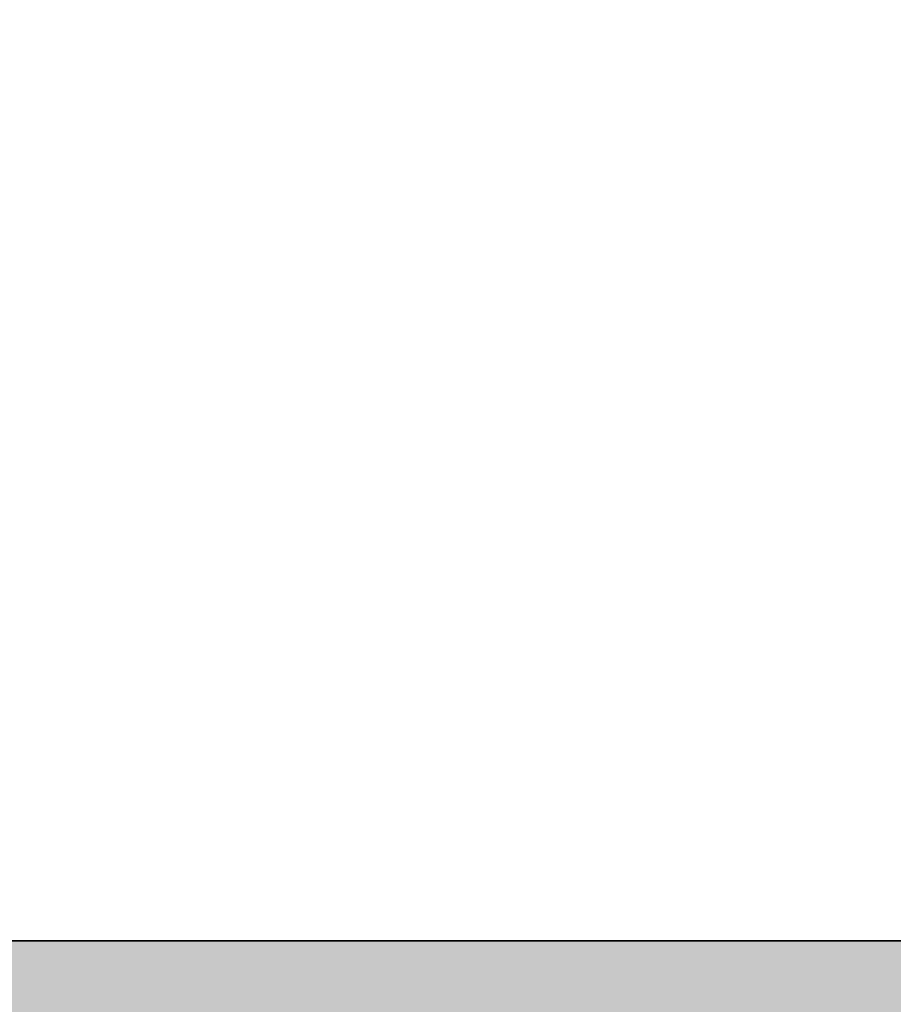
# Model space of a CAD drawing. Units: inches. Extents: x 2083 to 3317, y 1141 to 2115.
# Tile 27 of 256: x 2235.9182 to 2235.95532, y 1477.75866 to 1477.8005. Entities that reach past the tile are written whole.
import ezdxf

# ---------------------------------------------------------------- set-up
doc = ezdxf.new("R2010")
doc.units = ezdxf.units.IN
doc.layers.add('A-ANNO-DIMS', color=2, linetype='Continuous', lineweight=18)
doc.layers.add('A-WALL', color=7, linetype='Continuous', lineweight=35)
doc.layers.add('A-WALL-PATT', color=251, linetype='Continuous', lineweight=13, true_color=0x636466)
doc.styles.get("Standard").update_dxf_attribs({"font": 'arial.ttf'})
doc.dimstyles.new('ISO-25', dxfattribs={"dimtxt": 12, "dimasz": 12, "dimexe": 1.25, "dimexo": 0.625, "dimtad": 1, "dimlunit": 3, "dimtxsty": 'Standard', "dimcen": 2.5, "dimadec": 0, "dimazin": 0, "dimtfac": 1, "dimtmove": 0, "dimatfit": 3, "dimfxl": 1, "dimarcsym": 0})

# ---------------------------------------------------------------- blocks, each defined once
blk = doc.blocks.new('*D30')
at = {"layer": 'A-ANNO-DIMS', "color": 0, "lineweight": -2, "transparency": 16777216}
for p, q in [((2240.017856, 1445.273807), (2240.017856, 1448.045528)), ((2254.329327, 1445.273807), (2254.329327, 1448.045528)), ((2228.017856, 1446.795528), (2216.017856, 1446.795528)), ((2240.017856, 1446.795528), (2254.329327, 1446.795528)), ((2266.329327, 1446.795528), (2413.764866, 1446.795528))]:
    blk.add_line(p, q, dxfattribs=at)
at = {"layer": 'A-ANNO-DIMS', "color": 0, "transparency": 16777216}
for points in [[(2228.017856, 1448.795528), (2228.017856, 1444.795528), (2240.017856, 1446.795528)], [(2266.329327, 1448.795528), (2266.329327, 1444.795528), (2254.329327, 1446.795528)]]:
    blk.add_solid(points, dxfattribs=at)
at = {"layer": 'Defpoints', "color": 0, "transparency": 16777216}
for p in [(2254.329327, 1446.795528), (2240.017856, 1444.648807), (2254.329327, 1444.648807)]:
    blk.add_point(p, dxfattribs=at)
at = {"layer": 'A-ANNO-DIMS', "color": 0, "transparency": 16777216, "insert": (2346.047096, 1453.625167), "char_height": 12, "attachment_point": 5}
blk.add_mtext('WC 1\'-2 1/2" TYP.', dxfattribs=at)
blk = doc.blocks.new('*D31')
at = {"layer": 'A-ANNO-DIMS', "color": 0, "lineweight": -2, "transparency": 16777216}
for p, q in [((2237.871136, 1456.648807), (2237.871136, 1541.915179)), ((2239.392856, 1444.648807), (2236.621136, 1444.648807)), ((2237.871136, 1431.547542), (2237.871136, 1444.648807)), ((2239.392856, 1431.547542), (2236.621136, 1431.547542)), ((2237.871136, 1419.547542), (2237.871136, 1407.547542))]:
    blk.add_line(p, q, dxfattribs=at)
at = {"layer": 'A-ANNO-DIMS', "color": 0, "transparency": 16777216}
for points in [[(2235.871136, 1456.648807), (2239.871136, 1456.648807), (2237.871136, 1444.648807)], [(2235.871136, 1419.547542), (2239.871136, 1419.547542), (2237.871136, 1431.547542)]]:
    blk.add_solid(points, dxfattribs=at)
at = {"layer": 'Defpoints', "color": 0, "transparency": 16777216}
for p in [(2237.871136, 1444.648807), (2240.017856, 1444.648807), (2240.017856, 1431.547542)]:
    blk.add_point(p, dxfattribs=at)
at = {"layer": 'A-ANNO-DIMS', "color": 0, "transparency": 16777216, "insert": (2231.217486, 1505.281993), "char_height": 12, "attachment_point": 5, "rotation": 90}
blk.add_mtext('1\'-1" TYP.', dxfattribs=at)

msp = doc.modelspace()

# ---------------------------------------------------------------- hatches: boundary and pattern name
at = {"layer": 'A-WALL-PATT'}
h = msp.add_hatch(color=256, dxfattribs=at)
h.dxf.hatch_style = 1
h.paths.add_polyline_path([(3126.959783, 2020.76136), (2748.959783, 2020.76136), (2604.959783, 2020.76136), (2226.959783, 2020.76136), (2226.959783, 1702.76136), (2466.959783, 1702.76136), (2466.959783, 1582.76136), (2418.959783, 1582.76136), (2418.959783, 1477.76136), (2226.959783, 1477.76136), (2226.959783, 1263.26136), (2544.959783, 1263.26136), (2544.959783, 1411.76136), (2604.959783, 1411.76136), (2685.959783, 1411.76136), (2685.959783, 1420.76136), (2604.959783, 1420.76136), (2604.959783, 1573.76136), (2604.959783, 1702.76136), (2604.959783, 2011.76136), (2748.959783, 2011.76136), (2748.959783, 1702.76136), (2862.959783, 1702.76136), (2862.959783, 1621.76136), (2871.959783, 1621.76136), (2871.959783, 1702.76136), (2883.959783, 1702.76136), (2883.959783, 1706.939459, -0.026459), (2883.959783, 1711.76136), (2757.959783, 1711.76136), (2757.959783, 1807.76136), (2787.959783, 1807.76136), (2787.959783, 1812.26136), (2757.959783, 1812.26136), (2757.959783, 2011.76136), (2877.959783, 2011.76136), (2877.959783, 1812.26136), (2847.959783, 1812.26136), (2847.959783, 1807.76136), (2889.835742, 1807.76136), (2889.835742, 1812.26136), (2882.459783, 1812.26136), (2882.459783, 2011.76136), (3117.959783, 2011.76136), (3117.959783, 1812.26136), (2937.835742, 1812.26136), (2937.835742, 1807.76136), (2995.709783, 1807.76136), (2995.709783, 1796.117666), (3000.209783, 1796.117666), (3000.209783, 1807.76136), (3117.959783, 1807.76136), (3117.959783, 1711.76136), (3000.209783, 1711.76136), (3000.209783, 1760.117666), (2998.572705, 1760.117666, -0.020711), (2995.709783, 1760.117666), (2995.709783, 1711.76136), (2931.959783, 1711.76136), (2931.959783, 1702.76136), (3126.959783, 1702.76136)])
h.paths.add_polyline_path([(2471.459783, 2011.76136), (2471.459783, 1810.01136), (2462.716936, 1810.01136), (2462.716936, 1805.51136), (2505.959783, 1805.51136), (2505.959783, 1810.01136), (2475.959783, 1810.01136), (2475.959783, 2011.76136), (2595.959783, 2011.76136), (2595.959783, 1810.01136), (2565.959783, 1810.01136), (2565.959783, 1805.51136), (2595.959783, 1805.51136), (2595.959783, 1711.76136), (2235.959783, 1711.76136), (2235.959783, 1805.51136), (2353.709783, 1805.51136), (2353.709783, 1796.054162), (2358.209783, 1796.054162), (2358.209783, 1805.51136), (2414.716936, 1805.51136), (2414.716936, 1810.01136), (2235.959783, 1810.01136), (2235.959783, 2011.76136)], flags=16)
h.paths.add_polyline_path([(2270.204734, 1994.610008), (2270.204734, 1970.610008), (2246.204734, 1970.610008), (2246.204734, 1994.610008)], flags=0)
edge = h.paths.add_edge_path(flags=0)
edge.add_ellipse((2332.027391, 1899.798176), major_axis=(-3.042994, 3.042994), ratio=0.16825245, start_angle=-161.332166, end_angle=-156.307114, ccw=False)
edge.add_ellipse((2333.082037, 1898.74353), major_axis=(-1.054646, 1.054646), ratio=0.4535321, start_angle=-123.371019, end_angle=-94.159107)
edge = h.paths.add_edge_path(flags=0)
edge.add_ellipse((2332.027391, 1968.87629), major_axis=(3.042994, 3.042994), ratio=0.16825245, start_angle=18.667834, end_angle=23.692886)
edge.add_spline(control_points=[(2332.925596, 1970.691105), (2332.226768, 1970.3361), (2330.893709, 1969.658905), (2328.41308, 1970.932138), (2327.203934, 1967.748712), (2324.709596, 1969.955589), (2322.532822, 1967.012354), (2320.012846, 1971.295812), (2317.680308, 1968.157845), (2316.040526, 1967.102047), (2315.426904, 1966.809602)], knot_values=[0, 0, 0, 0, 2.267059, 4.324559, 6.685584, 8.878641, 11.121502, 14.300359, 17.755284, 19.732645, 19.732645, 19.732645, 19.732645], degree=3, periodic=0)
edge.add_ellipse((2332.027391, 1968.87629), major_axis=(3.042994, 3.042994), ratio=0.16825245, start_angle=18.667834, end_angle=23.692886, ccw=False)
edge.add_ellipse((2333.082037, 1969.930936), major_axis=(1.054646, 1.054646), ratio=0.4535321, start_angle=56.628981, end_angle=85.840893, ccw=False)
edge = h.paths.add_edge_path(flags=0)
edge.add_spline(control_points=[(2296.428287, 1967.987908), (2293.627804, 1965.336314), (2287.703624, 1959.727094), (2299.74386, 1949.995699), (2294.532591, 1935.668528), (2290.573228, 1920.603512), (2293.394124, 1909.973691), (2296.185407, 1904.966543)], knot_values=[0.099185, 0.099185, 0.099185, 0.099185, 0.345301, 0.619822, 0.982653, 1.386093, 1.810555, 1.810555, 1.810555, 1.810555], degree=3, periodic=0)
edge.add_spline(control_points=[(2296.185407, 1904.966543), (2297.383582, 1902.6193), (2298.000969, 1901.949312), (2298.55297, 1901.468155)], knot_values=[0.006246, 0.006246, 0.006246, 0.006246, 0.055476, 0.055476, 0.055476, 0.055476], degree=3, periodic=0)
edge.add_spline(control_points=[(2298.55297, 1901.468155), (2297.258612, 1900.923224), (2295.225294, 1900.232126), (2293.060229, 1900.614205), (2292.101423, 1900.788415), (2292.089578, 1900.790568)], knot_values=[0.312835, 0.312835, 0.312835, 0.312835, 0.40178, 0.474987, 0.475903, 0.475903, 0.475903, 0.475903], degree=3, periodic=0)
edge.add_arc((2292.793646, 1904.664109), 3.937008, 215.420897, 259.698179, ccw=False)
edge.add_spline(control_points=[(2289.585314, 1902.382304), (2289.476652, 1902.535087), (2289.36848, 1902.688035), (2289.260865, 1902.84117)], knot_values=[0.102872, 0.102872, 0.102872, 0.102872, 0.116896, 0.116896, 0.116896, 0.116896], degree=3, periodic=0)
edge.add_spline(control_points=[(2289.260865, 1902.84117), (2288.686604, 1902.550192), (2287.640048, 1902.019902), (2285.881337, 1901.873954), (2283.852972, 1901.504352), (2281.719987, 1899.710538), (2278.466991, 1899.492942), (2276.157136, 1901.883202), (2272.258953, 1899.804071), (2267.777605, 1901.843183), (2262.243882, 1900.184033), (2257.414927, 1901.782061), (2254.318374, 1900.72612), (2253.178285, 1900.337343)], knot_values=[0, 0, 0, 0, 1.907977, 3.477176, 5.261074, 7.972851, 11.680248, 13.717921, 16.939592, 22.789562, 27.502503, 33.595215, 37.145618, 37.145618, 37.145618, 37.145618], degree=3, periodic=0)
edge.add_line((2253.178285, 1900.337343), (2250.24424, 1902.84117))
edge.add_line((2250.24424, 1902.84117), (2250.24424, 1965.833296))
edge.add_line((2250.24424, 1965.833296), (2253.178285, 1968.337123))
edge.add_spline(control_points=[(2253.178285, 1968.337123), (2254.318374, 1967.948346), (2257.414927, 1966.892405), (2262.243882, 1968.490433), (2267.777605, 1966.831283), (2271.52673, 1968.537217), (2273.875914, 1967.828289), (2274.206701, 1967.727642)], knot_values=[0, 0, 0, 0, 0.09018, 0.244935, 0.364644, 0.513233, 0.537855, 0.537855, 0.537855, 0.537855], degree=3, periodic=0)
edge.add_arc((2274.352887, 1963.793349), 3.937008, 72.051134, 92.127949, ccw=False)
edge.add_arc((2281.296933, 1985.230003), 18.596298, 252.0511336, 288.5657217)
edge.add_arc((2292.316717, 1956.02888), 12.646081, 71.0267879, 113.7782184, ccw=False)
edge = h.paths.add_edge_path(flags=0)
edge.add_spline(control_points=[(2274.899415, 1951.856195), (2275.066156, 1951.616592), (2275.232687, 1951.376588), (2275.397987, 1951.135855)], knot_values=[1.409916, 1.409916, 1.409916, 1.409916, 1.43159, 1.43159, 1.43159, 1.43159], degree=3, periodic=0)
edge.add_spline(control_points=[(2275.397987, 1951.135855), (2275.792106, 1950.561885), (2276.179231, 1949.983774), (2276.545546, 1949.397103)], knot_values=[1.358238, 1.358238, 1.358238, 1.358238, 1.409916, 1.409916, 1.409916, 1.409916], degree=3, periodic=0)
edge.add_line((2276.545546, 1949.397103), (2277.437289, 1947.862185))
edge.add_spline(control_points=[(2277.437289, 1947.862185), (2276.303834, 1945.673115), (2274.639698, 1942.426882), (2274.631615, 1938.0939), (2272.799124, 1930.85155), (2274.356426, 1943.897046), (2275.947681, 1947.923356), (2276.545546, 1949.397103)], knot_values=[0.005632, 0.005632, 0.005632, 0.005632, 0.186014, 0.266002, 0.357087, 0.59639, 0.739732, 0.739732, 0.739732, 0.739732], degree=3, periodic=0)
edge.add_spline(control_points=[(2276.545546, 1949.397103), (2276.179231, 1949.983774), (2275.792106, 1950.561885), (2275.397987, 1951.135855)], knot_values=[1.358238, 1.358238, 1.358238, 1.358238, 1.409916, 1.409916, 1.409916, 1.409916], degree=3, periodic=0)
edge.add_spline(control_points=[(2275.397987, 1951.135855), (2274.9425, 1950.080452), (2274.20776, 1948.025272), (2273.934602, 1944.851477), (2272.468534, 1937.627489), (2273.466216, 1945.696466), (2274.700615, 1951.059472), (2274.899415, 1951.856195)], knot_values=[0.104364, 0.104364, 0.104364, 0.104364, 0.189636, 0.269624, 0.36071, 0.600013, 0.644622, 0.644622, 0.644622, 0.644622], degree=3, periodic=0)
h.paths.add_polyline_path([(2269.167514, 1963.127573, -0.357527), (2268.170633, 1960.97637, -0.092561), (2268.170633, 1939.436325, -0.357527), (2269.167514, 1937.285122, -0.357527), (2267.01631, 1938.282002, -0.164785), (2254.685581, 1938.282002, -0.357527), (2252.534378, 1937.285122, -0.357527), (2253.531259, 1939.436325, -0.092561), (2253.531259, 1960.97637, -0.357527), (2252.534378, 1963.127573, -0.357527), (2254.685581, 1962.130692, -0.164785), (2267.01631, 1962.130692, -0.357527)], flags=0)
h.paths.add_polyline_path([(2248.874068, 1967.8018), (2248.874068, 1957.02771), (2249.457783, 1957.02771), (2249.457783, 1911.646756), (2248.874068, 1911.646756), (2248.874068, 1900.872666), (2246.511863, 1900.872666, 0.197327), (2244.149658, 1902.456873), (2244.149658, 1966.217592, 0.197327), (2246.511863, 1967.8018)], flags=0)
h.paths.add_polyline_path([(2269.167514, 1931.389344, -0.357527), (2268.170633, 1929.238141, -0.092561), (2268.170633, 1907.698096, -0.357527), (2269.167514, 1905.546893, -0.357527), (2267.01631, 1906.543774, -0.164785), (2254.685581, 1906.543774, -0.357527), (2252.534378, 1905.546893, -0.357527), (2253.531259, 1907.698096, -0.092561), (2253.531259, 1929.238141, -0.357527), (2252.534378, 1931.389344, -0.357527), (2254.685581, 1930.392463, -0.164785), (2267.01631, 1930.392463, -0.357527)], flags=0)
edge = h.paths.add_edge_path(flags=0)
edge.add_spline(control_points=[(2276.196858, 1906.723702), (2276.168144, 1909.028928), (2276.114049, 1913.371852), (2270.598417, 1924.924978), (2273.905175, 1919.012779), (2275.921711, 1916.262063), (2275.47457, 1912.402149), (2277.257874, 1910.380621), (2276.696044, 1908.225036), (2276.646218, 1906.813023), (2276.617825, 1906.008407)], knot_values=[0, 0, 0, 0, 8.61026, 16.221274, 18.843057, 23.804898, 27.440828, 29.356102, 31.203478, 33.650687, 33.650687, 33.650687, 33.650687], degree=3, periodic=0)
edge.add_spline(control_points=[(2276.617825, 1906.008407), (2276.623313, 1905.624144), (2276.497738, 1904.628661), (2275.441779, 1903.854725), (2274.937314, 1903.08045), (2274.85908, 1902.84117)], knot_values=[0.156488, 0.156488, 0.156488, 0.156488, 0.184398, 0.231376, 0.250598, 0.250598, 0.250598, 0.250598], degree=3, periodic=0)
edge.add_line((2274.85908, 1902.84117), (2276.50598, 1902.84117))
edge.add_spline(control_points=[(2276.50598, 1902.84117), (2276.788308, 1903.08494), (2277.665071, 1904.125196), (2278.249538, 1904.340738), (2277.653872, 1908.527387), (2278.15567, 1906.227808), (2278.100464, 1905.285948), (2278.846675, 1904.069005), (2277.856785, 1903.414948), (2277.874191, 1902.99105), (2277.903562, 1902.84117)], knot_values=[0.059574, 0.059574, 0.059574, 0.059574, 0.080753, 0.103741, 0.16972, 0.176036, 0.207137, 0.240474, 0.262341, 0.27366, 0.27366, 0.27366, 0.27366], degree=3, periodic=0)
edge.add_line((2277.903562, 1902.84117), (2280.029825, 1902.84117))
edge.add_spline(control_points=[(2280.029825, 1902.84117), (2279.888221, 1903.088398), (2279.499257, 1903.981551), (2280.152284, 1905.939349), (2278.103615, 1909.657757), (2279.762395, 1907.185285), (2280.3279, 1904.874861), (2280.485109, 1903.48959), (2281.463269, 1903.249432), (2281.758343, 1902.936497), (2281.834036, 1902.84117)], knot_values=[0.013856, 0.013856, 0.013856, 0.013856, 0.034874, 0.088867, 0.107879, 0.126738, 0.158714, 0.193757, 0.217487, 0.226722, 0.226722, 0.226722, 0.226722], degree=3, periodic=0)
edge.add_spline(control_points=[(2281.834036, 1902.84117), (2281.787535, 1902.826703), (2281.647022, 1902.782988), (2281.395527, 1902.85949), (2281.088077, 1902.985242), (2280.720683, 1903.060902), (2280.333451, 1903.025726), (2280.124767, 1902.898879), (2280.029825, 1902.84117)], knot_values=[0, 0, 0, 0, 0.14413, 0.435517, 0.749276, 1.153046, 1.548371, 1.878348, 1.878348, 1.878348, 1.878348], degree=3, periodic=0)
edge.add_line((2280.029825, 1902.84117), (2277.903562, 1902.84117))
edge.add_spline(control_points=[(2277.903562, 1902.84117), (2277.892855, 1902.795855), (2277.865396, 1902.679637), (2277.607479, 1902.687483), (2277.27405, 1902.8007), (2276.837921, 1902.619775), (2276.583807, 1902.789261), (2276.50598, 1902.84117)], knot_values=[0, 0, 0, 0, 0.127189, 0.326199, 0.628009, 1.24357, 1.515331, 1.515331, 1.515331, 1.515331], degree=3, periodic=0)
edge.add_line((2276.50598, 1902.84117), (2274.85908, 1902.84117))
edge.add_spline(control_points=[(2274.85908, 1902.84117), (2274.814437, 1902.898587), (2274.72513, 1903.013446), (2274.493477, 1903.118968), (2274.244285, 1902.960539), (2273.937121, 1903.184942), (2273.614039, 1902.983143), (2273.408316, 1902.883045), (2273.322254, 1902.84117)], knot_values=[0, 0, 0, 0, 0.21843, 0.436957, 0.687977, 0.990379, 1.398396, 1.69185, 1.69185, 1.69185, 1.69185], degree=3, periodic=0)
edge.add_spline(control_points=[(2273.322254, 1902.84117), (2273.61674, 1903.445692), (2274.273998, 1904.538253), (2276.027239, 1904.573702), (2276.206963, 1906.583637), (2276.196858, 1906.723702)], knot_values=[0.012227, 0.012227, 0.012227, 0.012227, 0.059472, 0.106218, 0.134458, 0.134458, 0.134458, 0.134458], degree=3, periodic=0)
h.paths.add_polyline_path([(2270.776054, 1897.789828), (2270.776054, 1873.789828), (2246.776054, 1873.789828), (2246.776054, 1897.789828)], flags=0)
h.paths.add_polyline_path([(2353.709783, 1760.005059), (2353.709783, 1760.054162), (2358.209783, 1760.054162, -0.033729)], flags=0)
h.paths.add_polyline_path([(2321.819119, 1737.529186), (2341.995327, 1737.529186, -0.414214), (2343.203273, 1736.321241), (2343.203273, 1721.020596, -0.414214), (2341.995327, 1719.812651), (2321.819119, 1719.812651, -0.414214), (2320.611173, 1721.020596), (2320.611173, 1736.321241, -0.414214)], flags=0)
h.paths.add_polyline_path([(2324.23501, 1736.321241), (2339.579436, 1736.321241, -0.414214), (2341.995327, 1733.905349), (2341.995327, 1725.44973, -0.414214), (2339.579436, 1723.033839), (2333.680588, 1723.033839), (2333.845317, 1722.045467, -0.870646), (2335.425399, 1721.825893, -0.767327), (2333.922694, 1721.423245), (2331.291024, 1721.423245, -0.767327), (2329.788319, 1721.825893, -0.870646), (2331.368401, 1722.045467), (2331.53313, 1723.033839), (2324.23501, 1723.033839, -0.414214), (2321.819119, 1725.44973), (2321.819119, 1733.905349, -0.414214)], flags=0)
h.paths.add_polyline_path([(2570.483789, 1928.615444), (2589.683789, 1928.615444), (2590.168829, 1928.615444), (2590.168829, 1904.993397), (2570.483789, 1904.993397)], flags=0)
h.paths.add_polyline_path([(2574.447324, 1927.263822, -1), (2572.828836, 1927.263822, -1)], flags=0)
h.paths.add_polyline_path([(2573.089867, 1926.940877), (2573.925032, 1927.776042), (2574.147743, 1927.553332), (2573.312577, 1926.718166)], flags=0)
h.paths.add_polyline_path([(2578.779065, 1919.729618, -1), (2571.591663, 1919.729618, -1)], flags=0)
h.paths.add_polyline_path([(2578.385364, 1919.729618, -1), (2571.985364, 1919.729618, -1)], flags=0)
h.paths.add_polyline_path([(2331.595764, 1729.476216, -1), (2333.617954, 1729.476216, -1)], flags=0)
h.paths.add_polyline_path([(2578.034228, 1927.263822, -1), (2576.41574, 1927.263822, -1)], flags=0)
h.paths.add_polyline_path([(2576.688851, 1927.531089), (2576.911562, 1927.753799), (2577.746728, 1926.918634), (2577.524017, 1926.695923)], flags=0)
h.paths.add_polyline_path([(2578.139065, 1909.859539, -1), (2572.231663, 1909.859539, -1)], flags=0)
h.paths.add_polyline_path([(2577.745364, 1909.859539, -1), (2572.625364, 1909.859539, -1)], flags=0)
h.paths.add_polyline_path([(2583.797718, 1927.263822, -1), (2582.179229, 1927.263822, -1)], flags=0)
h.paths.add_polyline_path([(2582.718649, 1927.753799), (2583.553814, 1926.918634), (2583.331103, 1926.695923), (2582.495938, 1927.531089)], flags=0)
h.paths.add_polyline_path([(2582.495938, 1927.531089), (2582.718649, 1927.753799), (2583.553814, 1926.918634), (2583.331103, 1926.695923)], flags=0)
h.paths.add_polyline_path([(2587.739065, 1920.529618, -1), (2581.831663, 1920.529618, -1)], flags=0)
h.paths.add_polyline_path([(2587.345364, 1920.529618, -1), (2582.225364, 1920.529618, -1)], flags=0)
h.paths.add_polyline_path([(2587.384622, 1927.263822, -1), (2585.766133, 1927.263822, -1)], flags=0)
h.paths.add_polyline_path([(2586.081993, 1926.980247), (2586.917158, 1927.815412), (2587.139869, 1927.592702), (2586.304703, 1926.757536)], flags=0)
h.paths.add_polyline_path([(2588.379065, 1910.659539, -1), (2581.191663, 1910.659539, -1)], flags=0)
h.paths.add_polyline_path([(2587.985364, 1910.659539, -1), (2581.585364, 1910.659539, -1)], flags=0)
h.paths.add_polyline_path([(2417.167729, 1729.477895), (2437.343937, 1729.477895, -0.414214), (2438.551883, 1728.26995), (2438.551883, 1712.969306, -0.414214), (2437.343937, 1711.76136), (2417.167729, 1711.76136, -0.414214), (2415.959783, 1712.969306), (2415.959783, 1728.26995, -0.414214)], flags=0)
h.paths.add_polyline_path([(2419.58362, 1728.26995), (2434.928046, 1728.26995, -0.414214), (2437.343937, 1725.854059), (2437.343937, 1717.39844, -0.414214), (2434.928046, 1714.982548), (2429.029199, 1714.982548), (2429.193927, 1713.994176, -0.870646), (2430.774009, 1713.774603, -0.767327), (2429.271304, 1713.371954), (2426.639634, 1713.371954, -0.767327), (2425.136929, 1713.774603, -0.870646), (2426.717011, 1713.994176), (2426.88174, 1714.982548), (2419.58362, 1714.982548, -0.414214), (2417.167729, 1717.39844), (2417.167729, 1725.854059, -0.414214)], flags=0)
h.paths.add_polyline_path([(2419.58362, 1728.26995), (2434.928046, 1728.26995, -0.414214), (2437.343937, 1725.854059), (2437.343937, 1717.39844, -0.414214), (2434.928046, 1714.982548), (2429.029199, 1714.982548), (2428.358118, 1719.009034), (2427.552821, 1719.009034), (2426.88174, 1714.982548), (2419.58362, 1714.982548, -0.414214), (2417.167729, 1717.39844), (2417.167729, 1725.854059, -0.414214)], flags=0)
h.paths.add_polyline_path([(2426.944374, 1721.424925, -1), (2428.966564, 1721.424925, -1)], flags=0)
h.paths.add_polyline_path([(2475.959783, 1702.76136), (2595.959783, 1702.76136), (2595.959783, 1582.76136), (2475.959783, 1582.76136)], flags=16)
h.paths.add_polyline_path([(2427.959783, 1573.76136), (2595.959783, 1573.76136), (2595.959783, 1468.76136), (2595.959783, 1420.76136), (2384.459783, 1420.76136), (2384.459783, 1468.76136), (2427.959783, 1468.76136)], flags=16)
h.paths.add_polyline_path([(2379.959783, 1468.76136), (2379.959783, 1420.76136), (2235.959783, 1420.76136), (2235.959783, 1468.76136)], flags=16)
h.paths.add_polyline_path([(2317.815996, 1466.695767), (2337.992205, 1466.695767, -0.414214), (2339.20015, 1465.487821), (2339.20015, 1450.187177, -0.414214), (2337.992205, 1448.979232), (2317.815996, 1448.979232, -0.414214), (2316.608051, 1450.187177), (2316.608051, 1465.487821, -0.414214)], flags=0)
h.paths.add_polyline_path([(2320.231887, 1465.487821), (2335.576313, 1465.487821, -0.414214), (2337.992205, 1463.07193), (2337.992205, 1454.616311, -0.414214), (2335.576313, 1452.20042), (2329.677466, 1452.20042), (2329.842195, 1451.212047, -0.870646), (2331.422276, 1450.992474, -0.767327), (2329.919571, 1450.589826), (2327.287902, 1450.589826, -0.767327), (2325.785197, 1450.992474, -0.870646), (2327.365278, 1451.212047), (2327.530007, 1452.20042), (2320.231887, 1452.20042, -0.414214), (2317.815996, 1454.616311), (2317.815996, 1463.07193, -0.414214)], flags=0)
h.paths.add_polyline_path([(2320.231887, 1465.487821), (2335.576313, 1465.487821, -0.414214), (2337.992205, 1463.07193), (2337.992205, 1454.616311, -0.414214), (2335.576313, 1452.20042), (2329.677466, 1452.20042), (2329.006385, 1456.226905), (2328.201088, 1456.226905), (2327.530007, 1452.20042), (2320.231887, 1452.20042, -0.414214), (2317.815996, 1454.616311), (2317.815996, 1463.07193, -0.414214)], flags=0)
h.paths.add_polyline_path([(2327.592641, 1458.642796, -1), (2329.614832, 1458.642796, -1)], flags=0)
h.paths.add_polyline_path([(2244.411744, 1433.340453), (2241.920945, 1433.340453, -0.414214), (2240.017856, 1435.243542), (2240.017856, 1440.952808, -0.414211), (2241.920925, 1442.855897), (2244.411744, 1442.855897, -1.976472)], flags=0)
h.paths.add_polyline_path([(2245.356888, 1434.397536, -0.414214), (2245.356888, 1441.798814, -2.144098)], flags=0)
h.paths.add_polyline_path([(2535.959783, 1416.26136), (2535.959783, 1272.26136), (2235.959783, 1272.26136), (2235.959783, 1416.26136)], flags=16)
h.paths.add_polyline_path([(2260.119561, 1384.292841), (2260.119561, 1362.038649), (2237.865369, 1362.038649), (2237.865369, 1384.292841)], flags=0)
edge = h.paths.add_edge_path(flags=0)
edge.add_line((2318.251847, 1362.093298), (2318.145797, 1362.000973))
edge.add_ellipse((2317.445116, 1360.431044), major_axis=(2.82164, 2.82164), ratio=0.16825245, start_angle=18.667834, end_angle=20.948127, ccw=False)
edge.add_ellipse((2318.423045, 1361.408974), major_axis=(0.977929, 0.977929), ratio=0.4535321, start_angle=56.628981, end_angle=70.226201, ccw=False)
edge = h.paths.add_edge_path(flags=0)
edge.add_line((2319.10737, 1295.571078), (2319.015044, 1295.677128))
edge.add_ellipse((2317.445116, 1296.377809), major_axis=(-2.82164, 2.82164), ratio=0.16825245, start_angle=-161.332166, end_angle=-159.051873, ccw=False)
edge.add_ellipse((2318.423045, 1295.39988), major_axis=(-0.977929, 0.977929), ratio=0.4535321, start_angle=-123.371019, end_angle=-109.773799)
edge = h.paths.add_edge_path(flags=0)
edge.add_spline(control_points=[(2284.210349, 1301.170219), (2284.580688, 1300.444719), (2284.891189, 1299.892024), (2285.159553, 1299.461018)], knot_values=[0.039066, 0.039066, 0.039066, 0.039066, 0.055476, 0.055476, 0.055476, 0.055476], degree=3, periodic=0)
edge.add_line((2285.159553, 1299.461018), (2284.210349, 1301.170219))
edge = h.paths.add_edge_path(flags=0)
edge.add_line((2280.412458, 1297.298013), (2283.369991, 1297.036122))
edge.add_line((2283.369991, 1297.036122), (2286.40569, 1297.92631))
edge.add_spline(control_points=[(2286.40569, 1297.92631), (2285.305487, 1297.463119), (2284.344777, 1297.129151), (2283.369991, 1297.036122)], knot_values=[0.394369, 0.394369, 0.394369, 0.394369, 0.475903, 0.475903, 0.475903, 0.475903], degree=3, periodic=0)
edge.add_spline(control_points=[(2283.369991, 1297.036122), (2283.28139, 1297.027666), (2282.316289, 1296.957336), (2281.312502, 1297.134479), (2280.423441, 1297.296016), (2280.412458, 1297.298013)], knot_values=[0.312835, 0.312835, 0.312835, 0.312835, 0.320246, 0.393453, 0.394369, 0.394369, 0.394369, 0.394369], degree=3, periodic=0)
edge = h.paths.add_edge_path(flags=0)
edge.add_line((2284.435561, 1359.607285), (2280.446291, 1355.328047))
edge.add_line((2280.446291, 1355.328047), (2279.579987, 1351.017754))
edge.add_line((2279.579987, 1351.017754), (2282.412974, 1346.580433))
edge.add_spline(control_points=[(2282.412974, 1346.580433), (2283.153331, 1345.589236), (2284.252896, 1344.028897), (2284.801037, 1342.387167), (2284.935162, 1341.805544)], knot_values=[1.240098, 1.240098, 1.240098, 1.240098, 1.332892, 1.382712, 1.382712, 1.382712, 1.382712], degree=3, periodic=0)
edge.add_spline(control_points=[(2284.935162, 1341.805544), (2285.319108, 1340.1406), (2285.233029, 1338.409204), (2284.909938, 1336.654122)], knot_values=[1.097484, 1.097484, 1.097484, 1.097484, 1.240098, 1.240098, 1.240098, 1.240098], degree=3, periodic=0)
edge.add_spline(control_points=[(2284.909938, 1336.654122), (2284.586848, 1334.89904), (2284.026745, 1333.120272), (2283.462644, 1331.360585)], knot_values=[0.95487, 0.95487, 0.95487, 0.95487, 1.097484, 1.097484, 1.097484, 1.097484], degree=3, periodic=0)
edge.add_line((2283.462644, 1331.360585), (2281.890376, 1326.153357))
edge.add_line((2281.890376, 1326.153357), (2280.756259, 1321.056089))
edge.add_line((2280.756259, 1321.056089), (2280.299205, 1316.001977))
edge.add_line((2280.299205, 1316.001977), (2280.715933, 1310.950068))
edge.add_line((2280.715933, 1310.950068), (2282.028094, 1305.972137))
edge.add_line((2282.028094, 1305.972137), (2284.210349, 1301.170219))
edge.add_spline(control_points=[(2284.210349, 1301.170219), (2283.340731, 1302.730185), (2282.611904, 1304.336493), (2282.028094, 1305.972137)], knot_values=[0.099185, 0.099185, 0.099185, 0.099185, 0.241799, 0.241799, 0.241799, 0.241799], degree=3, periodic=0)
edge.add_spline(control_points=[(2282.028094, 1305.972137), (2281.444283, 1307.60778), (2281.005489, 1309.272759), (2280.715933, 1310.950068)], knot_values=[0.241799, 0.241799, 0.241799, 0.241799, 0.384413, 0.384413, 0.384413, 0.384413], degree=3, periodic=0)
edge.add_spline(control_points=[(2280.715933, 1310.950068), (2280.433241, 1312.587613), (2280.289386, 1314.276959), (2280.298894, 1315.962032), (2280.299205, 1316.001977)], knot_values=[0.384413, 0.384413, 0.384413, 0.384413, 0.523647, 0.527028, 0.527028, 0.527028, 0.527028], degree=3, periodic=0)
edge.add_spline(control_points=[(2280.299205, 1316.001977), (2280.312326, 1317.686955), (2280.477871, 1319.367926), (2280.756259, 1321.056089)], knot_values=[0.527028, 0.527028, 0.527028, 0.527028, 0.669642, 0.669642, 0.669642, 0.669642], degree=3, periodic=0)
edge.add_spline(control_points=[(2280.756259, 1321.056089), (2281.034648, 1322.744252), (2281.42588, 1324.439608), (2281.890376, 1326.153357)], knot_values=[0.669642, 0.669642, 0.669642, 0.669642, 0.812256, 0.812256, 0.812256, 0.812256], degree=3, periodic=0)
edge.add_spline(control_points=[(2281.890376, 1326.153357), (2282.264383, 1327.533251), (2282.78787, 1329.26181), (2283.352751, 1331.01778), (2283.462644, 1331.360585)], knot_values=[0.812256, 0.812256, 0.812256, 0.812256, 0.927087, 0.95487, 0.95487, 0.95487, 0.95487], degree=3, periodic=0)
edge.add_line((2283.462644, 1331.360585), (2284.909938, 1336.654122))
edge.add_line((2284.909938, 1336.654122), (2284.935162, 1341.805544))
edge.add_line((2284.935162, 1341.805544), (2282.412974, 1346.580433))
edge.add_spline(control_points=[(2282.412974, 1346.580433), (2281.275127, 1348.103792), (2280.078447, 1349.570318), (2279.579987, 1351.017754)], knot_values=[1.382712, 1.382712, 1.382712, 1.382712, 1.525326, 1.525326, 1.525326, 1.525326], degree=3, periodic=0)
edge.add_spline(control_points=[(2279.579987, 1351.017754), (2279.443282, 1351.414721), (2279.136312, 1352.856922), (2279.73519, 1354.290385), (2280.446291, 1355.328047)], knot_values=[1.525326, 1.525326, 1.525326, 1.525326, 1.564439, 1.667941, 1.667941, 1.667941, 1.667941], degree=3, periodic=0)
edge.add_spline(control_points=[(2280.446291, 1355.328047), (2281.426113, 1356.757835), (2282.930837, 1358.18256), (2284.435561, 1359.607285)], knot_values=[1.667941, 1.667941, 1.667941, 1.667941, 1.810555, 1.810555, 1.810555, 1.810555], degree=3, periodic=0)
edge.add_arc((2280.623075, 1348.518181), 11.72618, 71.0267879, 113.7782184)
edge.add_arc((2270.404892, 1375.595156), 17.243567, 252.0511336, 288.5657217, ccw=False)
edge.add_arc((2263.965969, 1355.717847), 3.650622, 72.051134, 92.127949)
edge.add_arc((2263.965969, 1355.717847), 3.650622, 92.127949, 177.98513)
edge.add_spline(control_points=[(2260.317604, 1355.846199), (2260.260417, 1354.220668), (2260.551278, 1350.186547), (2262.999344, 1346.766251), (2264.472741, 1344.649024)], knot_values=[1.43159, 1.43159, 1.43159, 1.43159, 1.564144, 1.770695, 1.770695, 1.770695, 1.770695], degree=3, periodic=0)
edge.add_line((2264.472741, 1344.649024), (2264.93559, 1343.98253))
edge.add_spline(control_points=[(2263.801044, 1340.248105), (2263.843238, 1340.514088), (2264.067244, 1341.756465), (2264.512693, 1343.002453), (2264.935047, 1343.981083)], knot_values=[0.53657, 0.53657, 0.53657, 0.53657, 0.559349, 0.644622, 0.644622, 0.644622, 0.644622], degree=3, periodic=0)
edge.add_spline(control_points=[(2264.935047, 1343.981083), (2265.117771, 1343.714975), (2265.298875, 1343.447906), (2265.476756, 1343.179365)], knot_values=[1.384077, 1.384077, 1.384077, 1.384077, 1.409916, 1.409916, 1.409916, 1.409916], degree=3, periodic=0)
edge.add_spline(control_points=[(2265.476756, 1343.179365), (2265.654637, 1342.910823), (2265.829296, 1342.64081), (2265.99913, 1342.368812)], knot_values=[1.358238, 1.358238, 1.358238, 1.358238, 1.384077, 1.384077, 1.384077, 1.384077], degree=3, periodic=0)
edge.add_line((2265.99913, 1342.368812), (2266.826006, 1340.945547))
edge.add_spline(control_points=[(2266.826006, 1340.945547), (2268.894401, 1337.089691), (2271.398173, 1325.843001), (2270.516164, 1310.568557), (2275.919376, 1301.860609), (2277.789511, 1299.19945)], knot_values=[0.116896, 0.116896, 0.116896, 0.116896, 0.472987, 1.050969, 1.313793, 1.313793, 1.313793, 1.313793], degree=3, periodic=0)
edge.add_spline(control_points=[(2277.789511, 1299.19945), (2277.839405, 1299.128452), (2277.889428, 1299.057498), (2277.939572, 1298.986584)], knot_values=[0.109884, 0.109884, 0.109884, 0.109884, 0.116896, 0.116896, 0.116896, 0.116896], degree=3, periodic=0)
edge.add_line((2277.939572, 1298.986584), (2277.788849, 1299.199114))
edge.add_spline(control_points=[(2277.788849, 1299.199114), (2277.256582, 1298.929414), (2276.28635, 1298.437902), (2275.039352, 1298.334419), (2274.38333, 1298.238895), (2274.215254, 1298.209338)], knot_values=[33.12187, 33.12187, 33.12187, 33.12187, 35.029056, 36.598255, 37.144827, 37.144827, 37.144827, 37.144827], degree=3, periodic=0)
edge.add_line((2274.215254, 1298.209338), (2273.073147, 1297.892961))
edge.add_spline(control_points=[(2273.073147, 1297.892961), (2272.322936, 1297.579784), (2271.039151, 1296.510508), (2269.248395, 1296.226062), (2268.4231, 1296.374654)], knot_values=[26.532584, 26.532584, 26.532584, 26.532584, 29.198919, 31.839101, 31.839101, 31.839101, 31.839101], degree=3, periodic=0)
edge.add_line((2268.4231, 1296.374654), (2263.878501, 1297.457534))
edge.add_spline(control_points=[(2263.878501, 1297.457534), (2263.556077, 1297.359435), (2261.860306, 1296.838694), (2260.23878, 1297.282407), (2258.933454, 1297.516461)], knot_values=[15.919551, 15.919551, 15.919551, 15.919551, 16.939592, 21.226067, 21.226067, 21.226067, 21.226067], degree=3, periodic=0)
edge.add_line((2258.933454, 1297.516461), (2254.055233, 1297.32901))
edge.add_spline(control_points=[(2254.055233, 1297.32901), (2253.755525, 1297.295815), (2252.113683, 1297.165174), (2250.461869, 1297.544221), (2249.129686, 1297.667882)], knot_values=[5.306517, 5.306517, 5.306517, 5.306517, 6.276435, 10.613034, 10.613034, 10.613034, 10.613034], degree=3, periodic=0)
edge.add_line((2249.129686, 1297.667882), (2244.33165, 1296.877756))
edge.add_line((2244.33165, 1296.877756), (2241.611033, 1299.19945))
edge.add_line((2241.611033, 1299.19945), (2241.611033, 1357.609404))
edge.add_line((2241.611033, 1357.609404), (2244.33165, 1359.931097))
edge.add_line((2244.33165, 1359.931097), (2252.728823, 1359.542692))
edge.add_spline(control_points=[(2252.728823, 1359.542692), (2252.870939, 1359.54644), (2253.30574, 1359.548172), (2253.739845, 1359.514274), (2254.031742, 1359.482426)], knot_values=[0.233291, 0.233291, 0.233291, 0.233291, 0.244935, 0.268927, 0.268927, 0.268927, 0.268927], degree=3, periodic=0)
edge.add_line((2254.031742, 1359.482426), (2259.58719, 1359.41639))
edge.add_spline(control_points=[(2259.58719, 1359.41639), (2260.677068, 1359.628503), (2262.073197, 1359.897003), (2263.523692, 1359.459278), (2263.830417, 1359.365952)], knot_values=[0.422516, 0.422516, 0.422516, 0.422516, 0.513233, 0.537855, 0.537855, 0.537855, 0.537855], degree=3, periodic=0)
edge.add_arc((2263.965969, 1355.717847), 3.650622, 72.051134, 92.127949, ccw=False)
edge.add_arc((2270.404892, 1375.595156), 17.243567, 252.0511336, 288.5657217)
edge.add_arc((2280.623075, 1348.518181), 11.72618, 71.0267879, 113.7782184, ccw=False)
h.paths.add_polyline_path([(2240.34053, 1359.434715), (2240.34053, 1349.444353), (2240.881785, 1349.444353), (2240.881785, 1307.3645), (2240.34053, 1307.3645), (2240.34053, 1297.374138), (2238.150157, 1297.374138, 0.197327), (2235.959783, 1298.843108), (2235.959783, 1357.965746, 0.197327), (2238.150157, 1359.434715)], flags=0)
h.paths.add_polyline_path([(2259.15779, 1355.1005, -0.357527), (2258.233425, 1353.10578, -0.092561), (2258.233425, 1333.132601, -0.357527), (2259.15779, 1331.13788, -0.357527), (2257.16307, 1332.062246, -0.164785), (2245.729302, 1332.062246, -0.357527), (2243.734582, 1331.13788, -0.357527), (2244.658947, 1333.132601, -0.092561), (2244.658947, 1353.10578, -0.357527), (2243.734582, 1355.1005, -0.357527), (2245.729302, 1354.176135, -0.164785), (2257.16307, 1354.176135, -0.357527)], flags=0)
edge = h.paths.add_edge_path(flags=0)
edge.add_line((2265.99913, 1342.368812), (2266.826006, 1340.945547))
edge.add_line((2266.826006, 1340.945547), (2265.307557, 1337.814066))
edge.add_line((2265.307557, 1337.814066), (2264.358232, 1334.652939))
edge.add_line((2264.358232, 1334.652939), (2264.262012, 1333.799705))
edge.add_spline(control_points=[(2264.262012, 1333.799705), (2264.208357, 1333.187055), (2264.16206, 1332.365525), (2264.007144, 1331.413933), (2263.969049, 1331.201834)], knot_values=[0.464444, 0.464444, 0.464444, 0.464444, 0.516691, 0.531608, 0.531608, 0.531608, 0.531608], degree=3, periodic=0)
edge.add_spline(control_points=[(2263.969049, 1331.201834), (2263.774535, 1330.118873), (2263.42437, 1328.790839), (2263.25742, 1328.530652), (2263.234028, 1328.514612)], knot_values=[0.372682, 0.372682, 0.372682, 0.372682, 0.44885, 0.464444, 0.464444, 0.464444, 0.464444], degree=3, periodic=0)
edge.add_spline(control_points=[(2263.234028, 1328.514612), (2263.096382, 1328.420227), (2263.13117, 1329.301477), (2263.274953, 1330.615749)], knot_values=[0.280919, 0.280919, 0.280919, 0.280919, 0.372682, 0.372682, 0.372682, 0.372682], degree=3, periodic=0)
edge.add_spline(control_points=[(2263.274953, 1330.615749), (2263.418736, 1331.930022), (2263.671515, 1333.677318), (2263.969852, 1335.315027)], knot_values=[0.189157, 0.189157, 0.189157, 0.189157, 0.280919, 0.280919, 0.280919, 0.280919], degree=3, periodic=0)
edge.add_spline(control_points=[(2263.969852, 1335.315027), (2264.100496, 1336.032192), (2264.418783, 1337.621911), (2264.754848, 1338.86443), (2264.947419, 1339.491124)], knot_values=[0.097394, 0.097394, 0.097394, 0.097394, 0.137578, 0.189157, 0.189157, 0.189157, 0.189157], degree=3, periodic=0)
edge.add_spline(control_points=[(2264.947419, 1339.491124), (2265.290017, 1340.606055), (2265.644238, 1341.493996), (2265.99913, 1342.368812)], knot_values=[0.005632, 0.005632, 0.005632, 0.005632, 0.097394, 0.097394, 0.097394, 0.097394], degree=3, periodic=0)
h.paths.add_polyline_path([(2259.15779, 1325.670973, -0.357527), (2258.233425, 1323.676253, -0.092561), (2258.233425, 1303.703073, -0.357527), (2259.15779, 1301.708353, -0.357527), (2257.16307, 1302.632719, -0.164785), (2245.729302, 1302.632719, -0.357527), (2243.734582, 1301.708353, -0.357527), (2244.658947, 1303.703073, -0.092561), (2244.658947, 1323.676253, -0.357527), (2243.734582, 1325.670973, -0.357527), (2245.729302, 1324.746608, -0.164785), (2257.16307, 1324.746608, -0.357527)], flags=0)
edge = h.paths.add_edge_path(flags=0)
edge.add_spline(control_points=[(2261.708938, 1317.311421), (2261.679482, 1317.41758), (2261.761858, 1317.388535), (2262.490736, 1316.089873), (2262.962185, 1315.300897)], knot_values=[14.955861, 14.955861, 14.955861, 14.955861, 16.221274, 18.694826, 18.694826, 18.694826, 18.694826], degree=3, periodic=0)
edge.add_spline(control_points=[(2262.962185, 1315.300897), (2262.990437, 1315.253617), (2263.702096, 1314.067376), (2264.348983, 1313.127153), (2264.730054, 1312.164154)], knot_values=[18.694826, 18.694826, 18.694826, 18.694826, 18.843057, 22.433791, 22.433791, 22.433791, 22.433791], degree=3, periodic=0)
edge.add_spline(control_points=[(2264.730054, 1312.164154), (2264.875565, 1311.796437), (2265.176873, 1310.769807), (2265.143069, 1309.559262), (2265.247736, 1308.824193)], knot_values=[22.433791, 22.433791, 22.433791, 22.433791, 23.804898, 26.172756, 26.172756, 26.172756, 26.172756], degree=3, periodic=0)
edge.add_line((2265.247736, 1308.824193), (2265.850774, 1307.171888))
edge.add_spline(control_points=[(2265.850774, 1307.171888), (2266.065025, 1306.821678), (2266.384387, 1306.332246), (2266.4244, 1305.780549), (2266.420369, 1305.611216)], knot_values=[28.062562, 28.062562, 28.062562, 28.062562, 29.356102, 29.911721, 29.911721, 29.911721, 29.911721], degree=3, periodic=0)
edge.add_spline(control_points=[(2266.420369, 1305.611216), (2266.416116, 1305.43259), (2266.393999, 1305.249998), (2266.364777, 1305.065857)], knot_values=[29.911721, 29.911721, 29.911721, 29.911721, 30.497837, 30.497837, 30.497837, 30.497837], degree=3, periodic=0)
edge.add_line((2266.364777, 1305.065857), (2266.066151, 1302.136295))
edge.add_spline(control_points=[(2266.066151, 1302.136295), (2266.07124, 1301.779984), (2265.998076, 1301.199985), (2265.663266, 1300.758961), (2265.508908, 1300.585882)], knot_values=[0.156488, 0.156488, 0.156488, 0.156488, 0.184398, 0.203543, 0.203543, 0.203543, 0.203543], degree=3, periodic=0)
edge.add_line((2265.508908, 1300.585882), (2264.435341, 1299.19945))
edge.add_line((2264.435341, 1299.19945), (2265.962442, 1299.19945))
edge.add_line((2265.962442, 1299.19945), (2267.33599, 1301.175276))
edge.add_line((2267.33599, 1301.175276), (2267.311667, 1301.986237))
edge.add_spline(control_points=[(2267.311667, 1301.986237), (2267.261111, 1302.862396), (2267.160212, 1303.737132), (2267.271486, 1303.325896)], knot_values=[0.126229, 0.126229, 0.126229, 0.126229, 0.166617, 0.166617, 0.166617, 0.166617], degree=3, periodic=0)
edge.add_spline(control_points=[(2267.271486, 1303.325896), (2267.280035, 1303.294305), (2267.309785, 1303.175366), (2267.37345, 1302.883608), (2267.406123, 1302.682829), (2267.417926, 1302.601025)], knot_values=[0.166617, 0.166617, 0.166617, 0.166617, 0.16972, 0.176036, 0.180765, 0.180765, 0.180765, 0.180765], degree=3, periodic=0)
edge.add_spline(control_points=[(2267.743891, 1300.987505), (2267.687583, 1301.150943), (2267.48052, 1301.656664), (2267.483751, 1302.144788), (2267.417926, 1302.601025)], knot_values=[0.180765, 0.180765, 0.180765, 0.180765, 0.193767, 0.220139, 0.220139, 0.220139, 0.220139], degree=3, periodic=0)
edge.add_line((2267.417926, 1302.601025), (2267.743891, 1300.987505))
edge.add_spline(control_points=[(2267.743891, 1300.987505), (2267.831961, 1300.731878), (2267.932021, 1300.309904), (2267.554841, 1299.974518), (2267.429366, 1299.829207)], knot_values=[0.220139, 0.220139, 0.220139, 0.220139, 0.240474, 0.25489, 0.25489, 0.25489, 0.25489], degree=3, periodic=0)
edge.add_line((2267.429366, 1299.829207), (2267.258361, 1299.19945))
edge.add_line((2267.258361, 1299.19945), (2269.229956, 1299.19945))
edge.add_spline(control_points=[(2269.229956, 1299.19945), (2269.098653, 1299.428694), (2268.842774, 1300.016251), (2269.011575, 1300.915923), (2268.946796, 1301.66074)], knot_values=[0.013856, 0.013856, 0.013856, 0.013856, 0.034874, 0.067073, 0.067073, 0.067073, 0.067073], degree=3, periodic=0)
edge.add_line((2268.946796, 1301.66074), (2268.431582, 1303.603109))
edge.add_spline(control_points=[(2268.431582, 1303.603109), (2268.175596, 1304.192375), (2267.596214, 1305.251298), (2268.040698, 1304.62321), (2268.251394, 1304.282421)], knot_values=[0.090155, 0.090155, 0.090155, 0.090155, 0.107879, 0.120289, 0.120289, 0.120289, 0.120289], degree=3, periodic=0)
edge.add_spline(control_points=[(2268.251394, 1304.282421), (2268.360882, 1304.105329), (2269.057753, 1302.917983), (2269.382691, 1301.590419), (2269.521405, 1300.775931), (2269.57522, 1300.555784)], knot_values=[0.120289, 0.120289, 0.120289, 0.120289, 0.126738, 0.158714, 0.173506, 0.173506, 0.173506, 0.173506], degree=3, periodic=0)
edge.add_line((2269.57522, 1300.555784), (2270.685798, 1299.421258))
edge.add_spline(control_points=[(2270.685798, 1299.421258), (2270.767221, 1299.357251), (2270.837852, 1299.281401), (2270.902925, 1299.19945)], knot_values=[0.21816, 0.21816, 0.21816, 0.21816, 0.226722, 0.226722, 0.226722, 0.226722], degree=3, periodic=0)
edge.add_line((2270.937201, 1299.192913), (2270.902925, 1299.19945))
edge.add_spline(control_points=[(2270.902925, 1299.19945), (2270.859806, 1299.186035), (2270.729515, 1299.1455), (2270.496314, 1299.216437), (2270.271661, 1299.308323), (2270.121017, 1299.347961), (2270.063339, 1299.359557)], knot_values=[0.939174, 0.939174, 0.939174, 0.939174, 1.083304, 1.374691, 1.68845, 1.878348, 1.878348, 1.878348, 1.878348], degree=3, periodic=0)
edge.add_line((2270.063339, 1299.359557), (2269.229956, 1299.19945))
edge.add_line((2269.229956, 1299.19945), (2267.258361, 1299.19945))
edge.add_spline(control_points=[(2267.258361, 1299.19945), (2267.248433, 1299.157431), (2267.222971, 1299.049667), (2266.983816, 1299.056942), (2266.80921, 1299.11623), (2266.676905, 1299.109091), (2266.636531, 1299.104815)], knot_values=[0.757665, 0.757665, 0.757665, 0.757665, 0.884854, 1.083864, 1.385675, 1.515331, 1.515331, 1.515331, 1.515331], degree=3, periodic=0)
edge.add_spline(control_points=[(2266.636531, 1299.104815), (2266.485225, 1299.088788), (2266.235807, 1299.017123), (2266.034608, 1299.151317), (2265.962442, 1299.19945)], knot_values=[0, 0, 0, 0, 0.485905, 0.757665, 0.757665, 0.757665, 0.757665], degree=3, periodic=0)
edge.add_line((2265.962442, 1299.19945), (2264.435341, 1299.19945))
edge.add_line((2264.435341, 1299.19945), (2263.858444, 1299.367118))
edge.add_spline(control_points=[(2263.858444, 1299.367118), (2263.818943, 1299.370905), (2263.779528, 1299.385721), (2263.740131, 1299.401504)], knot_values=[0.845925, 0.845925, 0.845925, 0.845925, 0.978627, 0.978627, 0.978627, 0.978627], degree=3, periodic=0)
edge.add_line((2263.721786, 1299.396425), (2263.010306, 1299.19945))
edge.add_spline(control_points=[(2263.010306, 1299.19945), (2263.245794, 1299.682859), (2263.506032, 1300.128107), (2263.873494, 1300.408028)], knot_values=[0.012227, 0.012227, 0.012227, 0.012227, 0.052971, 0.052971, 0.052971, 0.052971], degree=3, periodic=0)
edge.add_spline(control_points=[(2263.873494, 1300.408028), (2263.932131, 1300.452695), (2264.084243, 1300.552979), (2264.255189, 1300.624223), (2264.359686, 1300.664747)], knot_values=[0.052971, 0.052971, 0.052971, 0.052971, 0.059472, 0.069086, 0.069086, 0.069086, 0.069086], degree=3, periodic=0)
edge.add_line((2264.359686, 1300.664747), (2265.1419, 1301.077774))
edge.add_line((2265.1419, 1301.077774), (2265.675806, 1302.799558))
edge.add_line((2265.675806, 1302.799558), (2265.5407, 1305.704066))
edge.add_line((2265.5407, 1305.704066), (2264.803073, 1309.327724))
edge.add_line((2264.803073, 1309.327724), (2263.040535, 1314.091791))
edge.add_spline(control_points=[(2263.040535, 1314.091791), (2262.383572, 1315.671438), (2261.795972, 1316.997749), (2261.708938, 1317.311421)], knot_values=[11.216896, 11.216896, 11.216896, 11.216896, 14.955861, 14.955861, 14.955861, 14.955861], degree=3, periodic=0)
h.paths.add_polyline_path([(2871.959783, 1416.26136), (2895.910047, 1416.26136), (2895.910047, 1420.76136), (2871.959783, 1420.76136), (2871.959783, 1501.76136), (2862.959783, 1501.76136), (2862.959783, 1420.76136), (2805.959783, 1420.76136), (2805.959783, 1411.76136), (2862.959783, 1411.76136), (2862.959783, 1263.26136), (3126.959783, 1263.26136), (3126.959783, 1411.76136), (3126.959783, 1486.76136), (2943.959783, 1486.76136), (2943.959783, 1477.76136), (2967.860311, 1477.76136), (2967.860311, 1420.76136), (2943.910047, 1420.76136), (2943.910047, 1416.26136), (3117.959783, 1416.26136), (3117.959783, 1420.76136), (2972.360311, 1420.76136), (2972.360311, 1477.76136), (3117.959783, 1477.76136), (3117.959783, 1420.76136), (3117.959783, 1272.26136), (2871.959783, 1272.26136)], flags=0)
h.paths.add_polyline_path([(2457.125626, 1485.942505), (2527.602651, 1485.942505), (2527.602651, 1537.635702), (2457.125626, 1537.635702)], flags=8)
h.paths.add_polyline_path([(2481.005058, 1609.981804), (2590.765818, 1609.981804), (2590.765818, 1682.003362), (2481.005058, 1682.003362)], flags=8)
h.paths.add_polyline_path([(2483.085022, 1729.126784), (2553.562048, 1729.126784), (2553.562048, 1780.81998), (2483.085022, 1780.81998)], flags=8)

# ---------------------------------------------------------------- linework, layer by layer
at = {"layer": 'A-WALL'}
msp.add_line((2226.959783, 1477.76136), (2418.959783, 1477.76136), dxfattribs=at)

# ---------------------------------------------------------------- dimensions: what is measured, and where the dimension line sits
at = {"layer": 'A-ANNO-DIMS'}
dim = msp.add_linear_dim(base=(2237.871136, 1444.648807), p1=(2240.017856, 1431.547542), p2=(2240.017856, 1444.648807), angle=90, text='<> TYP.', dimstyle='ISO-25', override={"dimdec": 1, "dimlfac": 1, "dimrnd": 0, "dimzin": 1, "dimdsep": 46, "dimlunit": 4, "dimfrac": 2}, dxfattribs=at)
dim.commit()
dim.dimension.update_dxf_attribs({"geometry": '*D31', "text_midpoint": (2231.217486, 1505.281993)})
dim = msp.add_linear_dim(base=(2254.329327, 1446.795528), p1=(2240.017856, 1444.648807), p2=(2254.329327, 1444.648807), text='WC <> TYP.', dimstyle='ISO-25', override={"dimdec": 1, "dimlfac": 1, "dimrnd": 0, "dimzin": 1, "dimdsep": 46, "dimlunit": 4, "dimfrac": 2}, dxfattribs=at)
dim.commit()
dim.dimension.update_dxf_attribs({"geometry": '*D30', "text_midpoint": (2346.047096, 1453.625167)})

doc.saveas('drawing.dxf')
